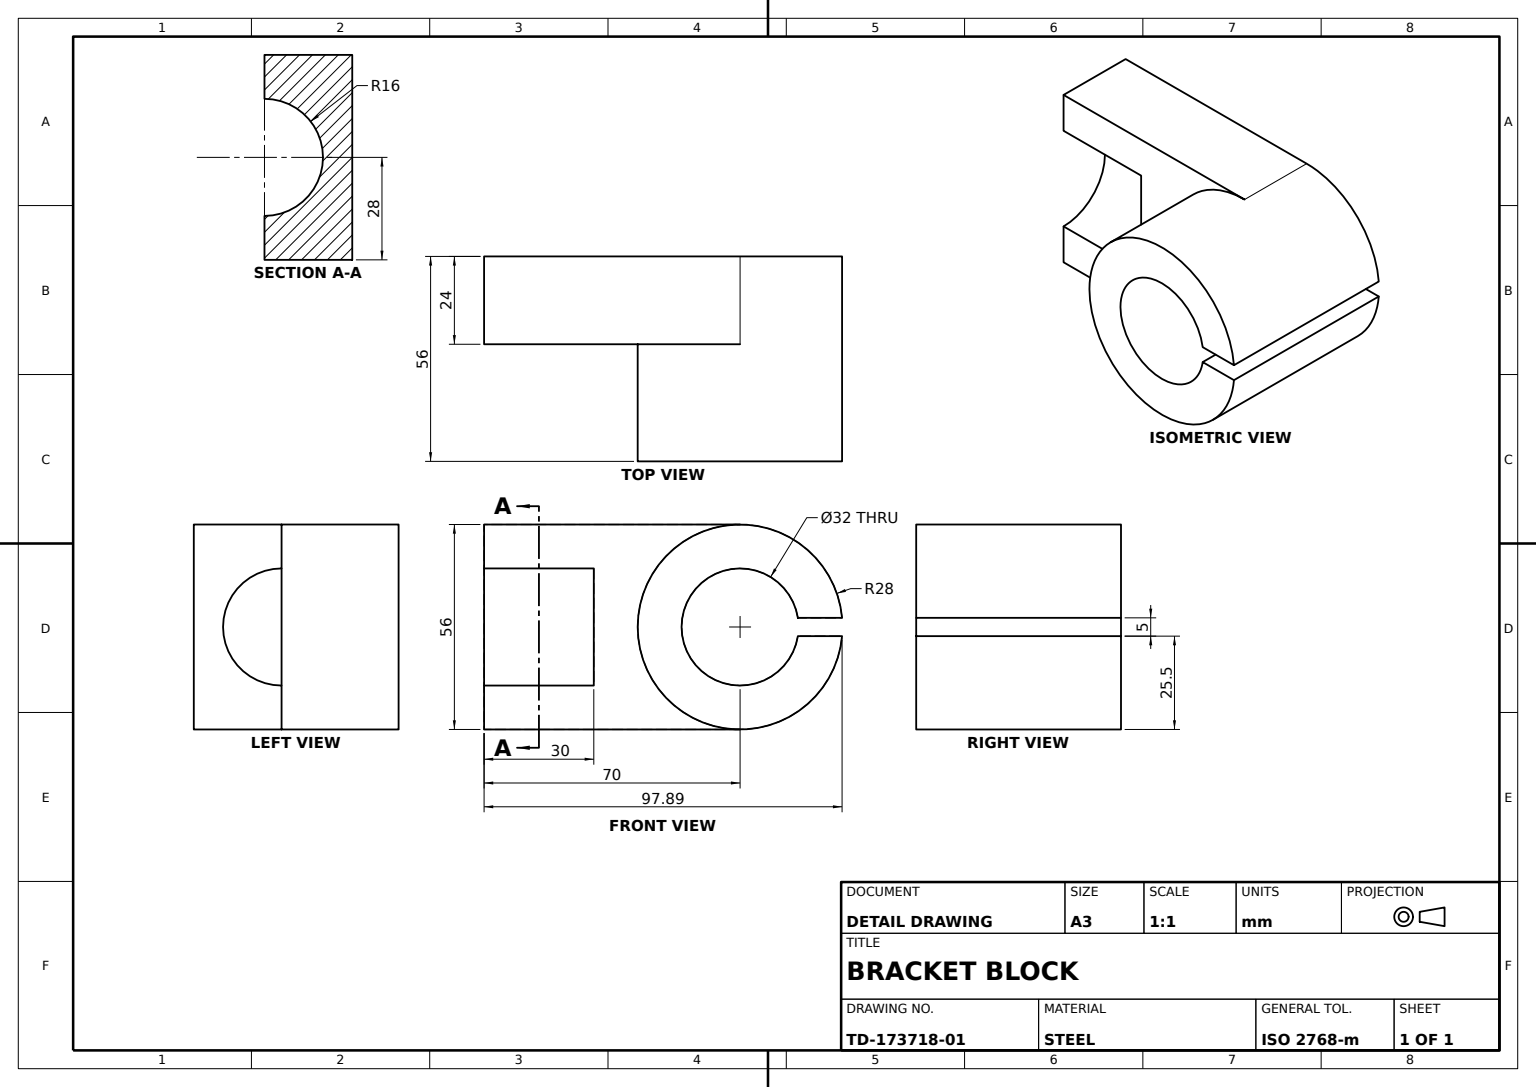
SolidWorks part; units mm, degrees
material "Plain Carbon Steel"
ref_plane "Front Plane" through (0, 0, 0) normal (0, 0, 1) x (1, 0, 0)
ref_plane "Top Plane" through (0, 0, 0) normal (0, 1, 0) x (1, 0, 0)
ref_plane "Right Plane" through (0, 0, 0) normal (1, 0, 0) x (0, 0, -1)
sketch "Base Block Sketch" plane through (0, 0, 0) normal (1, 0, 0) x (0, 0, -1)
  circle A0 centre (0, 0) radius 28
  circle A1 centre (0, 0) radius 16
  dimension "D1" = 56
  dimension "D2" = 32
extrude "Base Block" add sketch "Base Block Sketch" along normal blind 56
sketch "Boss Reference Line" plane through (0, 0, 0) normal (-1, 0, 0) x (0, 0, 1)
  line L0 (0, 0) -> (0, 28)
  circle A0 centre (0, 0) radius 28 construction
sketch "Clamp Boss Sketch" plane through (0, 0, 0) normal (-1, 0, 0) x (0, 0, 1)
  line L0 (0, 0) -> (0, 28)
  line L1 (0, 0) -> (0, -28)
  line L2 (0, 28) -> (70, 28)
  line L3 (70, 28) -> (70, -28)
  line L4 (70, -28) -> (0, -28)
  circle A0 centre (0, 0) radius 28 construction
  dimension "D1" = 70
extrude "Clamp Boss" add sketch "Clamp Boss Sketch" against normal blind 24
sketch "Side Window Sketch" plane through (0, 0, 0) normal (-1, 0, 0) x (0, 0, 1)
  line L0 (0, 16) -> (0, -16) construction
  line L1 (0, 16) -> (0, -16)
  arc A0 (0, -16) -> (0, 16) centre (0, 0) ccw
extrude "Side Window Cut" cut sketch "Side Window Sketch" against normal blind 54
sketch "Bore Sketch" plane through (0, 0, 70) normal (0, 0, 1) x (1, 0, 0)
  line L0 (24, -28) -> (24, 28) construction
  line L1 (24, 16) -> (24, -16)
  arc A0 (24, 16) -> (24, -16) centre (24, 0) ccw
  dimension "D1" = 32
extrude "Bore" cut sketch "Bore Sketch" against normal blind 30
sketch "Clamp Slit Sketch" plane through (56, 0, 0) normal (1, 0, 0) x (0, 0, -1)
  line L0 (28, 0) -> (30.1407, 0)
  line L6 (30.1407, 0) -> (30.1407, 2.5)
  line L7 (30.1407, 2.5) -> (15.8035, 2.5)
  line L8 (15.8035, 2.5) -> (15.8035, -2.5)
  line L9 (15.8035, -2.5) -> (30.1407, -2.5)
  line L10 (30.1407, -2.5) -> (30.1407, 0)
  circle A2 centre (0, 0) radius 28 construction
  circle A3 centre (0, 0) radius 16 construction
  circle M4 centre (0, 0) radius 28
  circle M5 centre (0, 0) radius 16
  dimension "D1" = 2.5
  dimension "D2" = 2.5
  dimension "D3" = 14.3373
extrude "Clamp Slit 2.5" cut sketch "Clamp Slit Sketch" against normal blind 80 contours L9 L7 M5 M4 | L9 L10 L0 M4 | L6 L7 L0 M4
